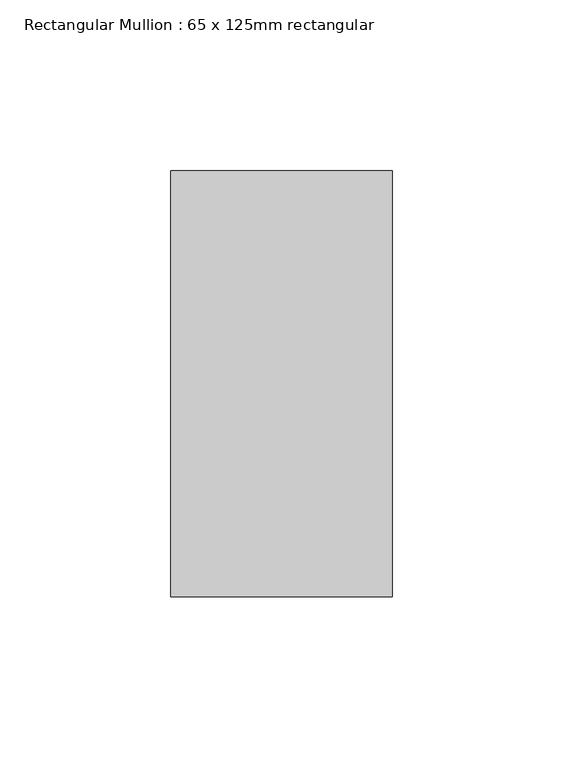
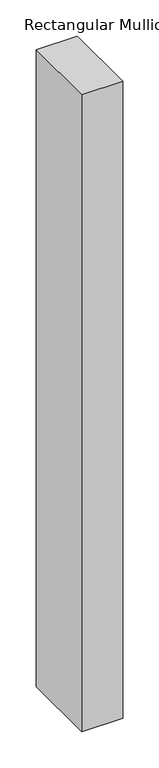
"""IFC4 building model written with IfcOpenShell, lengths in millimetres: member geometry, Rectangular Mullion : 65 x 125mm rectangular."""

from ifc_helpers import new_model, si_unit, frame, origin, place, context, project, spatial, polyline, outline, extrude, source, transform, mapped, element, save


def rectangular_mullion_65_x_125mm_rectangular_b7ff14d5(model_context):
    return source(origin(), model_context, "Body", "SweptSolid", [
        extrude(outline(polyline([(0.0, 62.5), (0.0, -62.5), (-65.0, -62.5), (-65.0, 62.5), (0.0, 62.5)])), frame((0.0, 0.0, -1070.0), z_axis=(0.0, 0.0, 1.0), x_axis=(1.0, 0.0, 0.0)), (0.0, 0.0, 1.0), 1070.0),
    ])


if __name__ == "__main__":
    model = new_model("IFC4")
    model_context = context("Model", 3, world=origin())
    ifc_project = project(units=[si_unit("LENGTHUNIT", "METRE", prefix="MILLI")], contexts=[model_context])
    site = spatial("IfcSite", under=ifc_project)
    building = spatial("IfcBuilding", under=site)
    placement = place(None, origin())
    rectangular_mullion_65_x_125mm_rectangular_shape = rectangular_mullion_65_x_125mm_rectangular_b7ff14d5(model_context)
    element("IfcMember", 1, ObjectType="Rectangular Mullion : 65 x 125mm rectangular", at=placement, inside=building, context=model_context, shape_type="MappedRepresentation", body=[
        mapped(rectangular_mullion_65_x_125mm_rectangular_shape, transform((0.0, 0.0, 0.0), x_axis=(1.0, 0.0, 0.0), y_axis=(0.0, 1.0, 0.0), z_axis=(0.0, 0.0, 1.0))),
    ])
    save(model, "model.ifc")

# Revit data of these elements
# Type "Rectangular Mullion : 65 x 125mm rectangular"
#   built-in parameter 1007304 = 0.410105 (stored number, unit not read)
#   built-in parameter 1007301 = 0.106627 (stored number, unit not read)
#   built-in parameter 1007300 = 0.106627 (stored number, unit not read)
# Element 1 (IfcMember, "Rectangular Mullion : 65 x 125mm rectangular")
#   Materials on its faces: "Aluminum"
# Materials
#   "Aluminum": class "Metal", colour RGB 244 245 246, transparency 0, Description = "Aluminum 6061", Cost = 0
